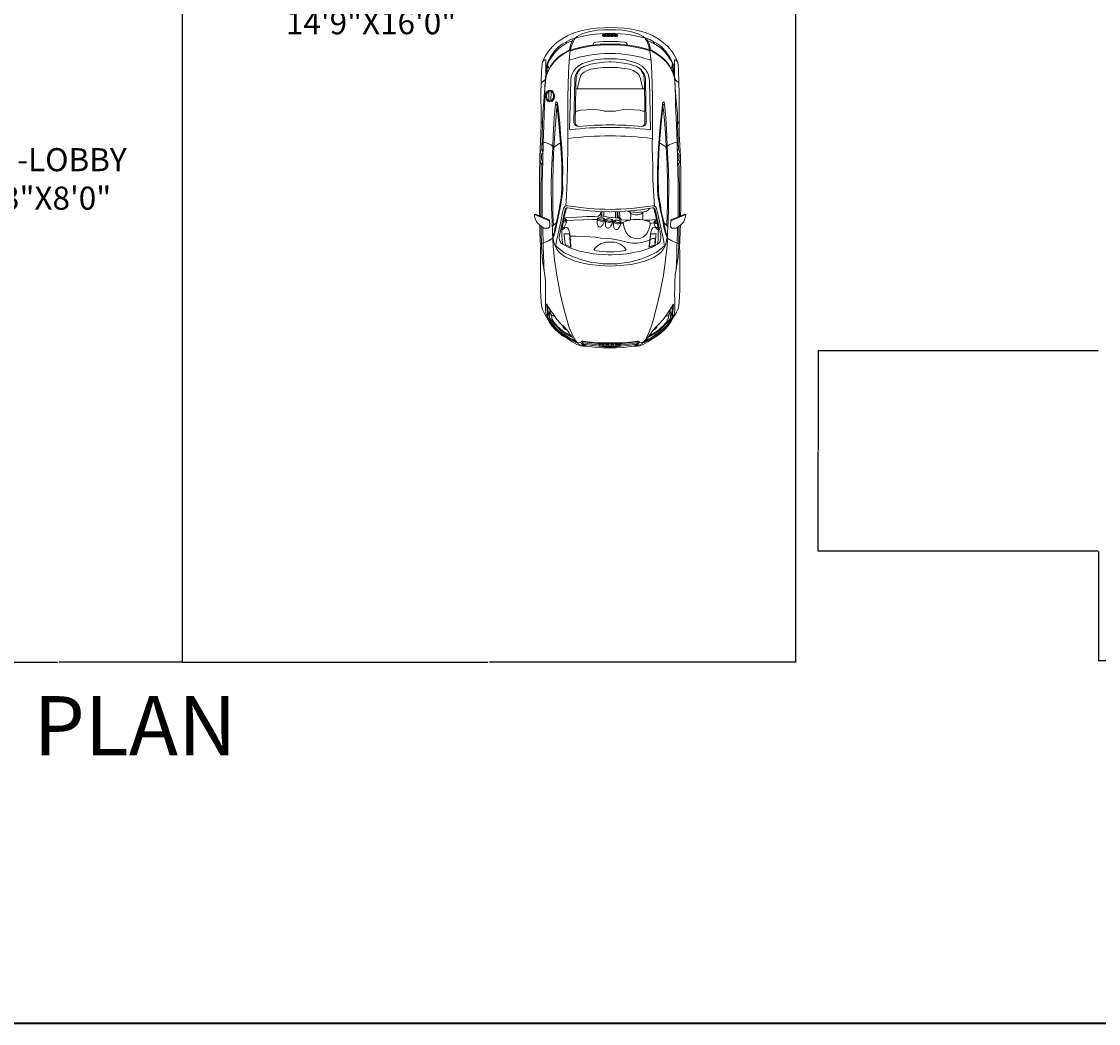
# Model space of a CAD drawing. Units: inches. Extents: x 2215 to 3724, y 1009 to 2124.
# Tile 5 of 11: x 2636 to 2963, y 1009 to 1313. Entities that reach past the tile are written whole.
import ezdxf

# ---------------------------------------------------------------- set-up
doc = ezdxf.new("R2010")
doc.units = ezdxf.units.IN
for name, color, linetype, lineweight in [('A-ANNO-DIMS', 2, 'Continuous', 18), ('A-ANNO-TEXT', 7, 'Continuous', 25), ('A-ANNO-TTLB', 7, 'Continuous', 35), ('A-AREA-IDEN', 7, 'Continuous', 18), ('AUDI', 8, 'Continuous', 13)]:
    doc.layers.add(name, color=color, linetype=linetype, lineweight=lineweight)
doc.styles.get("Standard").update_dxf_attribs({"font": 'arial.ttf'})
doc.dimstyles.get("Standard").update_dxf_attribs({"dimtxt": 0.18, "dimasz": 0.18, "dimexe": 0.18, "dimexo": 0.0625, "dimgap": 0.09, "dimtad": 0, "dimtih": 1, "dimtoh": 1, "dimdec": 4, "dimzin": 0, "dimdsep": 46, "dimtxsty": 'Standard', "dimcen": 0.09, "dimadec": 0, "dimazin": 0, "dimtfac": 1, "dimtdec": 4, "dimtofl": 0, "dimtmove": 0, "dimatfit": 3, "dimfxl": 1, "dimtolj": 1, "dimtzin": 0, "dimarcsym": 0})

# ---------------------------------------------------------------- blocks, each defined once
blk = doc.blocks.new('*D89')
at = {"layer": 'A-ANNO-DIMS', "color": 0, "lineweight": -2, "transparency": 16777216}
for p, q in [((2962.68, 1212.83), (2877.61, 1212.83)), ((2877.79, 1212.65), (2877.79, 1182.6)), ((2877.79, 1152.18), (2877.79, 1182.23)), ((2962.68, 1152), (2877.61, 1152))]:
    blk.add_line(p, q, dxfattribs=at)
at = {"layer": 'A-ANNO-DIMS', "color": 0, "transparency": 16777216}
for points in [[(2877.76, 1212.65), (2877.82, 1212.65), (2877.79, 1212.83)], [(2877.76, 1152.18), (2877.82, 1152.18), (2877.79, 1152)]]:
    blk.add_solid(points, dxfattribs=at)
at = {"layer": 'Defpoints', "color": 0, "transparency": 16777216}
for p in [(2877.79, 1212.83), (2962.74, 1212.83), (2962.74, 1152)]:
    blk.add_point(p, dxfattribs=at)
at = {"layer": 'A-ANNO-DIMS', "color": 0, "transparency": 16777216, "insert": (2877.79, 1182.42), "char_height": 0.18, "attachment_point": 5}
blk.add_mtext('\\A1;60.84', dxfattribs=at)
blk = doc.blocks.new('*D96')
at = {"layer": 'A-ANNO-DIMS', "color": 0, "lineweight": -2, "transparency": 16777216}
for p, q in [((3520.74, 1343.93), (3520.74, 1118.67)), ((2962.74, 1151.93), (2962.74, 1118.67)), ((2962.92, 1118.85), (3241.45, 1118.85)), ((3520.56, 1118.85), (3242.03, 1118.85))]:
    blk.add_line(p, q, dxfattribs=at)
at = {"layer": 'A-ANNO-DIMS', "color": 0, "transparency": 16777216}
for points in [[(2962.92, 1118.88), (2962.92, 1118.82), (2962.74, 1118.85)], [(3520.56, 1118.88), (3520.56, 1118.82), (3520.74, 1118.85)]]:
    blk.add_solid(points, dxfattribs=at)
at = {"layer": 'Defpoints', "color": 0, "transparency": 16777216}
for p in [(3520.74, 1344), (2962.74, 1152), (3520.74, 1118.85)]:
    blk.add_point(p, dxfattribs=at)
at = {"layer": 'A-ANNO-DIMS', "color": 0, "transparency": 16777216, "insert": (3241.74, 1118.85), "char_height": 0.18, "attachment_point": 5}
blk.add_mtext('\\A1;558', dxfattribs=at)
blk = doc.blocks.new('*D99')
at = {"layer": 'A-ANNO-DIMS', "color": 0, "lineweight": -2, "transparency": 16777216}
for p, q in [((2684.84, 1343.93), (2684.84, 1118.22)), ((2609.84, 1151.93), (2609.84, 1118.22)), ((2610.02, 1118.4), (2647.12, 1118.4)), ((2684.66, 1118.4), (2647.56, 1118.4))]:
    blk.add_line(p, q, dxfattribs=at)
at = {"layer": 'A-ANNO-DIMS', "color": 0, "transparency": 16777216}
for points in [[(2610.02, 1118.43), (2610.02, 1118.37), (2609.84, 1118.4)], [(2684.66, 1118.43), (2684.66, 1118.37), (2684.84, 1118.4)]]:
    blk.add_solid(points, dxfattribs=at)
at = {"layer": 'Defpoints', "color": 0, "transparency": 16777216}
for p in [(2684.84, 1344), (2609.84, 1152), (2684.84, 1118.4)]:
    blk.add_point(p, dxfattribs=at)
at = {"layer": 'A-ANNO-DIMS', "color": 0, "transparency": 16777216, "insert": (2647.34, 1118.4), "char_height": 0.18, "attachment_point": 5}
blk.add_mtext('\\A1;75', dxfattribs=at)
blk = doc.blocks.new('*D100')
at = {"layer": 'A-ANNO-DIMS', "color": 0, "lineweight": -2, "transparency": 16777216}
for p, q in [((2684.84, 1343.93), (2684.84, 1118.22)), ((2870.84, 1343.93), (2870.84, 1118.22)), ((2685.02, 1118.4), (2777.56, 1118.4)), ((2870.66, 1118.4), (2778.12, 1118.4))]:
    blk.add_line(p, q, dxfattribs=at)
at = {"layer": 'A-ANNO-DIMS', "color": 0, "transparency": 16777216}
for points in [[(2685.02, 1118.43), (2685.02, 1118.37), (2684.84, 1118.4)], [(2870.66, 1118.43), (2870.66, 1118.37), (2870.84, 1118.4)]]:
    blk.add_solid(points, dxfattribs=at)
at = {"layer": 'Defpoints', "color": 0, "transparency": 16777216}
for p in [(2684.84, 1344), (2870.84, 1344), (2870.84, 1118.4)]:
    blk.add_point(p, dxfattribs=at)
at = {"layer": 'A-ANNO-DIMS', "color": 0, "transparency": 16777216, "insert": (2777.84, 1118.4), "char_height": 0.18, "attachment_point": 5}
blk.add_mtext('\\A1;186', dxfattribs=at)

msp = doc.modelspace()

# ---------------------------------------------------------------- linework, layer by layer
at = {"layer": 'A-ANNO-TTLB'}
msp.add_lwpolyline([(2215.4438, 2124.2681), (3723.6589, 2124.2681), (3723.6589, 1008.7935), (2215.4438, 1008.7935)], close=True, dxfattribs=at)
at = {"layer": 'AUDI'}
for p, q in [((2801.1681, 1305.8265), (2801.323, 1306.5094)), ((2801.4616, 1305.9823), (2801.4475, 1306.5799)), ((2812.3228, 1308.4102), (2812.3228, 1308.6185)), ((2813.5649, 1308.1989), (2813.5649, 1308.4072)), ((2815.7326, 1308.1989), (2815.7326, 1308.4072)), ((2816.9747, 1308.4102), (2816.9747, 1308.6185)), ((2827.8359, 1305.9823), (2827.85, 1306.5799)), ((2828.1294, 1305.8265), (2827.9745, 1306.5094)), ((2804.207, 1292.2283), (2825.0905, 1292.2283)), ((2812.784, 1253.5837), (2812.784, 1255.0226)), ((2816.3282, 1253.0788), (2816.3282, 1255.0178)), ((2817.6075, 1253.179), (2817.377, 1253.179)), ((2826.7535, 1251.4199), (2827.33, 1251.5172)), ((2827.33, 1251.5172), (2828.0282, 1251.5961)), ((2813.1321, 1215.0864), (2813.1321, 1214.8065)), ((2816.0447, 1215.0864), (2816.0447, 1214.8065)), ((2811.4631, 1214.8025), (2811.4631, 1214.5226)), ((2817.7136, 1214.8025), (2817.7136, 1214.5226))]:
    msp.add_line(p, q, dxfattribs=at)
for points in [[(2793.2574, 1253.7096), (2793.2029, 1256.0458), (2793.2029, 1265.8842), (2793.3349, 1271.6287), (2793.6648, 1278.6278), (2793.738, 1281.6587), (2793.738, 1284.4076), (2793.677, 1290.7609), (2793.7685, 1294.304), (2793.8906, 1297.6944), (2794.0127, 1299.7409), (2794.1653, 1300.4435, -0.12683503), (2798.5051, 1306.2746), (2800.0673, 1307.3982), (2801.8248, 1308.4241), (2803.7288, 1309.2058), (2805.0469, 1309.5966), (2806.6579, 1310.0363), (2808.8059, 1310.4271), (2810.5146, 1310.6713), (2814.6488, 1310.8132)], [(2801.2318, 1256.7223), (2801.4068, 1259.7563), (2801.661, 1264.6858), (2801.6928, 1269.1383), (2801.8835, 1274.1632), (2801.8199, 1279.22), (2801.8296, 1289.7659), (2802.0096, 1297.0083), (2802.2323, 1300.7293), (2802.4772, 1303.0689), (2802.6524, 1304.072, -0.10917638), (2804.1487, 1307.7084), (2804.6219, 1308.1481), (2806.1132, 1308.9155), (2808.4993, 1309.6617), (2810.928, 1310.0241), (2812.7815, 1310.1094), (2814.6488, 1310.1094)], [(2836.0402, 1253.7096), (2836.0946, 1256.0458), (2836.0946, 1265.8842), (2835.9626, 1271.6287), (2835.6327, 1278.6278), (2835.5595, 1281.6587), (2835.5595, 1284.4076), (2835.6206, 1290.7609), (2835.529, 1294.304), (2835.4069, 1297.6944), (2835.2848, 1299.7409), (2835.1322, 1300.4435, 0.12683503), (2830.7924, 1306.2746), (2829.2302, 1307.3982), (2827.4727, 1308.4241), (2825.5688, 1309.2058), (2824.2507, 1309.5966), (2822.6396, 1310.0363), (2820.4916, 1310.4271), (2818.7829, 1310.6713), (2814.6488, 1310.8132)], [(2828.0815, 1256.4487), (2827.8908, 1259.7563), (2827.6365, 1264.6858), (2827.6047, 1269.1383), (2827.414, 1274.1632), (2827.4776, 1279.22), (2827.468, 1289.7659), (2827.2879, 1297.0083), (2827.0652, 1300.7293), (2826.8203, 1303.0689), (2826.6451, 1304.072, 0.10917638), (2825.1488, 1307.7084), (2824.6757, 1308.1481), (2823.1843, 1308.9155), (2820.7982, 1309.6617), (2818.3695, 1310.0241), (2816.516, 1310.1094), (2814.6488, 1310.1094)], [(2828.0657, 1256.7223), (2827.8908, 1259.7563), (2827.6365, 1264.6858), (2827.6047, 1269.1383), (2827.414, 1274.1632), (2827.4776, 1279.22), (2827.468, 1289.7659), (2827.2879, 1297.0083), (2827.0652, 1300.7293), (2826.8203, 1303.0689), (2826.6451, 1304.072, 0.10917638), (2825.1488, 1307.7084), (2824.6757, 1308.1481), (2823.1843, 1308.9155), (2820.7982, 1309.6617), (2818.3695, 1310.0241), (2816.516, 1310.1094), (2814.6488, 1310.1094)], [(2802.6416, 1307.2132, -0.1536904), (2826.6529, 1307.2309)], [(2810.3678, 1306.4047, -0.05356625), (2818.9097, 1306.4131, -0.05356625)], [(2802.603, 1303.7893, -0.14863541), (2826.6914, 1303.8068)], [(2802.6416, 1304.01, -0.1536904), (2826.6529, 1304.0276)], [(2802.2669, 1300.8894, -0.16706429), (2827.0472, 1300.9013, -0.16706429)], [(2802.5474, 1279.8089, -0.4622712), (2802.3789, 1280.0174), (2802.7384, 1294.8022, -0.18047602), (2804.1724, 1298.3779), (2804.9717, 1299.1307), (2806.2882, 1299.9305), (2808.2395, 1300.5421), (2810.0261, 1301.0597), (2812.7105, 1301.3722), (2814.6488, 1301.3722)], [(2805.0527, 1280.8316, -0.40402709), (2803.6614, 1282.0372), (2803.9118, 1294.9627, -0.22167644), (2805.5552, 1298.3163, -0.05999808), (2806.6597, 1299.0072), (2808.7671, 1299.718), (2810.4955, 1300.0734), (2812.816, 1300.334), (2814.3314, 1300.3814), (2814.6488, 1300.3814)], [(2826.7501, 1279.8089, 0.4622712), (2826.9186, 1280.0174), (2826.5592, 1294.8022, 0.18047602), (2825.1251, 1298.3779), (2824.3258, 1299.1307), (2823.0093, 1299.9305), (2821.0581, 1300.5421), (2819.2714, 1301.0597), (2816.5871, 1301.3722), (2814.6488, 1301.3722)], [(2824.2448, 1280.8316, 0.40402709), (2825.6361, 1282.0372), (2825.3858, 1294.9627, 0.22167644), (2823.7423, 1298.3163, 0.05999808), (2822.6378, 1299.0072), (2820.5305, 1299.718), (2818.802, 1300.0734), (2816.4816, 1300.334), (2814.9662, 1300.3814), (2814.6488, 1300.3814)], [(2805.9218, 1298.5875, 0.17077992), (2804.3629, 1295.619), (2804.2209, 1293.1548), (2804.1262, 1286.8287), (2804.0773, 1282.1936, 0.32699174), (2805.0527, 1280.8316, 1.80630344)], [(2808.7835, 1298.1873, -0.05874602), (2814.6488, 1298.7307, -0.04602302)], [(2820.5141, 1298.1873, 0.05874602), (2814.6488, 1298.7307, 0.04602302)], [(2823.3757, 1298.5875, -0.17077992), (2824.9346, 1295.619), (2825.0767, 1293.1548), (2825.1714, 1286.8287), (2825.2203, 1282.1936, -0.32699174), (2824.2448, 1280.8316, -1.80630344)], [(2802.5474, 1279.8089, -0.0615843), (2826.7583, 1279.8093, -0.0615843)], [(2805.0527, 1280.8316, -0.04880378), (2824.2662, 1280.8307, -0.04880378)], [(2801.8461, 1277.141, -0.06516086), (2827.4515, 1277.1425, -4.49164968)], [(2794.0848, 1269.347), (2794.1591, 1270.5362), (2794.1591, 1270.5362), (2794.0319, 1270.5275), (2793.9329, 1270.6018), (2793.8586, 1270.8248, -0.17711693), (2793.9081, 1272.5342), (2794.0113, 1272.6168), (2794.1459, 1272.6956), (2794.1459, 1272.6956), (2794.2086, 1272.7411), (2794.1839, 1273.3605), (2794.1096, 1273.8808), (2793.8338, 1273.8225), (2793.7638, 1273.6805, 0.20734628), (2793.7885, 1269.4937), (2793.809, 1269.4374), (2793.9824, 1269.3136), (2794.0848, 1269.347)], [(2835.2127, 1269.347), (2835.1384, 1270.5362), (2835.1384, 1270.5362), (2835.2656, 1270.5275), (2835.3647, 1270.6018), (2835.439, 1270.8248, 0.17711693), (2835.3894, 1272.5342), (2835.2862, 1272.6168), (2835.1517, 1272.6956), (2835.1517, 1272.6956), (2835.0889, 1272.7411), (2835.1137, 1273.3605), (2835.188, 1273.8808), (2835.4637, 1273.8225), (2835.5337, 1273.6805, -0.20734628), (2835.509, 1269.4937), (2835.4885, 1269.4374), (2835.3151, 1269.3136), (2835.2127, 1269.347)], [(2798.1177, 1244.3211), (2798.4791, 1246.5332), (2799.0555, 1249.1864), (2799.7759, 1252.474), (2800.2659, 1254.6945), (2800.5541, 1255.9346, -0.36424732), (2801.7068, 1256.7997, 0.04353666), (2814.6488, 1255.6808)], [(2814.6488, 1241.9147), (2814.0256, 1241.9147), (2811.5597, 1242.0028), (2809.5341, 1242.2231), (2807.5525, 1242.5756), (2805.3389, 1243.0544), (2803.5544, 1243.5969), (2802.1313, 1244.1393), (2800.8663, 1244.7949), (2800.2338, 1245.1565), (2799.8272, 1245.4504), (2799.4884, 1245.9025), (2799.3302, 1246.4224), (2799.2399, 1247.0101), (2799.2625, 1247.8464), (2800.9793, 1255.5995, -0.41343093), (2801.7925, 1256.1194), (2802.9967, 1255.9594), (2805.4544, 1255.5616), (2808.6349, 1255.2361), (2811.5263, 1255.0553), (2814.3093, 1254.9829)], [(2831.1798, 1244.3211), (2830.8185, 1246.5332), (2830.2421, 1249.1864), (2829.5216, 1252.474), (2829.0317, 1254.6945), (2828.7435, 1255.9346, 0.36424732), (2827.5907, 1256.7997, -0.04353666), (2814.6488, 1255.6808)], [(2814.6488, 1241.9147), (2815.2719, 1241.9147), (2817.7379, 1242.0028), (2819.7635, 1242.2231), (2821.7451, 1242.5756), (2823.9586, 1243.0544), (2825.7431, 1243.5969), (2827.1662, 1244.1393), (2828.4312, 1244.7949), (2829.0637, 1245.1565), (2829.4703, 1245.4504), (2829.8092, 1245.9025), (2829.9673, 1246.4224), (2830.0576, 1247.0101), (2830.035, 1247.8464), (2828.3183, 1255.5995, 0.41343093), (2827.5051, 1256.1194), (2826.3008, 1255.9594), (2823.8431, 1255.5616), (2820.6626, 1255.2361), (2817.7712, 1255.0553), (2814.9882, 1254.9829)], [(2819.8124, 1255.1829), (2820.1661, 1255.0256, 0.09257149), (2825.552, 1255.0256), (2826.1747, 1255.4617), (2826.6536, 1256.0063)], [(2822.6407, 1254.0124, -0.11496238), (2821.068, 1254.3714), (2820.6633, 1254.7141), (2820.5953, 1254.952)], [(2822.6407, 1254.0124, 0.11496238), (2824.2133, 1254.3714), (2824.618, 1254.7141), (2824.6678, 1254.8882)], [(2800.1147, 1250.0559, 0.30781353), (2800.8353, 1250.464), (2801.076, 1250.8446), (2801.3322, 1251.4676), (2801.4175, 1251.9726), (2801.4719, 1252.375), (2801.4665, 1252.5116), (2801.318, 1252.7381, 0.10075057), (2800.6404, 1252.9063, 0.03883263)], [(2810.7936, 1252.7669), (2810.7655, 1252.4293), (2810.7515, 1251.9791), (2810.7655, 1251.4726), (2810.8358, 1250.9661, 0.69697601), (2812.1856, 1250.6706), (2812.4668, 1251.0223), (2812.7901, 1251.6133), (2812.9307, 1252.1057), (2813.0292, 1252.4996), (2813.0389, 1252.636), (2812.7761, 1252.978, 0.1146222), (2811.2295, 1253.1609), (2811.0327, 1253.0764), (2810.8499, 1252.9357), (2810.7936, 1252.7669)], [(2813.2485, 1252.4241), (2813.2204, 1252.0865), (2813.2064, 1251.6363), (2813.2204, 1251.1298), (2813.2907, 1250.6233, 0.69697601), (2814.6405, 1250.3279), (2814.9217, 1250.6796), (2815.245, 1251.2705), (2815.3856, 1251.7629), (2815.4841, 1252.1568), (2815.4938, 1252.2932), (2815.231, 1252.6352, 0.1146222), (2813.6844, 1252.8181), (2813.4876, 1252.7337), (2813.3048, 1252.593), (2813.2485, 1252.4241)], [(2815.7546, 1251.9833), (2815.7265, 1251.6456), (2815.7124, 1251.1954), (2815.7265, 1250.689), (2815.7968, 1250.1825, 0.69697601), (2817.1465, 1249.887), (2817.4277, 1250.2387), (2817.7511, 1250.8296), (2817.8917, 1251.3221), (2817.9901, 1251.716), (2817.9998, 1251.8524), (2817.737, 1252.1944, 0.1146222), (2816.1904, 1252.3773), (2815.9936, 1252.2928), (2815.8108, 1252.1521), (2815.7546, 1251.9833)], [(2818.5801, 1251.7302), (2818.6793, 1250.9607), (2819.0018, 1249.8437), (2819.5475, 1248.7019, 0.61645483), (2826.0961, 1248.9253), (2826.5178, 1249.8686), (2826.7659, 1250.9111), (2826.7411, 1251.9287, 0.20084491), (2818.5801, 1251.7302, 3.44889889)], [(2829.124, 1250.3307, -0.43942644), (2828.5577, 1250.1994), (2828.3282, 1250.4647), (2828.1346, 1250.9355), (2828.0492, 1251.4405), (2827.9948, 1251.8429), (2828.0002, 1251.9795), (2828.1487, 1252.206, -0.09128884), (2828.7608, 1252.3702, -0.09128884)], [(2802.4871, 1247.6), (2804.1652, 1247.6), (2807.023, 1247.4833), (2810.2308, 1247.2498), (2812.3887, 1246.8996), (2815.0716, 1246.7246), (2817.7544, 1246.1993), (2819.3292, 1245.7908, 0.12760018), (2824.9865, 1245.7908), (2826.248, 1246.2818), (2826.8913, 1246.5577), (2827.5039, 1246.8182), (2827.9021, 1246.8948), (2828.1624, 1246.8948), (2828.2696, 1246.6343), (2828.2006, 1245.3967)], [(2814.6488, 1242.8529), (2813.5471, 1242.8529), (2811.3476, 1242.9718), (2810.5512, 1243.1377), (2810.0676, 1243.2399), (2809.8861, 1243.367), (2809.8316, 1243.4942), (2809.8679, 1243.6486, -0.25546602), (2814.6488, 1245.7741, -2.79521639)], [(2814.6488, 1242.8529), (2815.7504, 1242.8529), (2817.95, 1242.9718), (2818.7463, 1243.1377), (2819.2299, 1243.2399), (2819.4115, 1243.367), (2819.4659, 1243.4942), (2819.4296, 1243.6486, 0.25546602), (2814.6488, 1245.7741, 2.79521639)], [(2800.2416, 1220.472, 0.27931409), (2801.6606, 1219.0017, 0.27931409)], [(2829.056, 1220.472, -0.27931409), (2827.637, 1219.0017, -0.27931409)]]:
    msp.add_lwpolyline(points, format="xyb", dxfattribs=at)
for points in [[(2802.6416, 1307.2132), (2801.5459, 1306.6356), (2800.0836, 1305.8074), (2798.9524, 1304.8411), (2797.7385, 1303.5987), (2796.6073, 1301.9146), (2795.9175, 1300.6447), (2795.5313, 1299.8716), (2795.3657, 1299.0158), (2795.3657, 1297.9391), (2795.3382, 1296.7243), (2795.3206, 1296.2338)], [(2803.2085, 1306.7744), (2802.37, 1306.4643), (2800.8669, 1305.6667), (2799.1588, 1304.5272), (2798.0656, 1303.4333), (2797.0635, 1302.1571), (2796.3575, 1301.0177), (2795.9704, 1300.3112), (2795.7654, 1299.7871), (2795.6743, 1299.1262), (2795.606, 1298.0323), (2795.606, 1297.2229)], [(2803.5853, 1307.4984), (2803.2565, 1306.8841), (2802.6771, 1305.5589), (2802.4564, 1304.5926), (2802.3309, 1304.04)], [(2810.3678, 1306.4047), (2809.7673, 1306.1511), (2809.5021, 1305.8193), (2809.4181, 1305.5168)], [(2814.6488, 1308.4261), (2814.6488, 1308.2178)], [(2818.9097, 1306.4131), (2819.5302, 1306.1511), (2819.7954, 1305.8193), (2819.8774, 1305.5241)], [(2825.7122, 1307.4984), (2826.041, 1306.8841), (2826.6204, 1305.5589), (2826.8411, 1304.5926), (2826.9667, 1304.04)], [(2826.089, 1306.7744), (2826.9276, 1306.4643), (2828.4307, 1305.6667), (2830.1388, 1304.5272), (2831.2319, 1303.4333), (2832.234, 1302.1571), (2832.94, 1301.0177), (2833.3272, 1300.3112), (2833.5321, 1299.7871), (2833.6232, 1299.1262), (2833.6915, 1298.0323), (2833.6915, 1297.2229)], [(2826.656, 1307.2132), (2827.7516, 1306.6356), (2829.2139, 1305.8074), (2830.3451, 1304.8411), (2831.559, 1303.5987), (2832.6902, 1301.9146), (2833.38, 1300.6447), (2833.7662, 1299.8716), (2833.9318, 1299.0158), (2833.9318, 1297.9391), (2833.9594, 1296.7243), (2833.9769, 1296.2338)], [(2802.3309, 1304.04), (2801.999, 1303.8657), (2800.4359, 1302.9951), (2798.9466, 1301.8737), (2797.6637, 1300.6194), (2796.5697, 1299.1071), (2795.6496, 1297.3128), (2795.3361, 1296.6656)], [(2802.6416, 1304.01), (2801.999, 1303.6724), (2800.4359, 1302.8018), (2798.9466, 1301.6804), (2797.6637, 1300.4262), (2796.5697, 1298.9138), (2795.6496, 1297.1195), (2795.4127, 1296.6305)], [(2826.656, 1304.01), (2827.2985, 1303.6724), (2828.8616, 1302.8018), (2830.3509, 1301.6804), (2831.6338, 1300.4262), (2832.7278, 1298.9138), (2833.648, 1297.1195), (2833.8848, 1296.6305)], [(2826.9667, 1304.04), (2827.2985, 1303.8657), (2828.8616, 1302.9951), (2830.3509, 1301.8737), (2831.6338, 1300.6194), (2832.7278, 1299.1071), (2833.648, 1297.3128), (2833.9615, 1296.6656)], [(2794.0225, 1253.3989), (2794.0225, 1259.1275), (2794.0225, 1263.7106), (2794.2045, 1270.4183), (2794.3562, 1275.8513), (2794.5601, 1281.2664), (2794.8027, 1287.2882), (2794.8351, 1289.1349), (2794.9036, 1293.0363), (2795.1268, 1296.5975), (2795.1208, 1298.8552), (2795.1247, 1300.5002)], [(2795.1247, 1300.5002), (2795.1198, 1300.9076), (2795.0199, 1301.0327), (2794.8325, 1301.0327), (2794.6826, 1300.9701), (2794.5202, 1300.8076), (2794.2953, 1300.5451), (2794.1482, 1300.3644)], [(2796.2643, 1298.3184), (2796.0387, 1298.6248), (2795.8565, 1298.9438), (2795.7882, 1299.3996), (2795.7654, 1300.0377), (2795.7978, 1300.405)], [(2833.0332, 1298.3184), (2833.2588, 1298.6248), (2833.441, 1298.9438), (2833.5094, 1299.3996), (2833.5321, 1300.0377), (2833.4997, 1300.405)], [(2835.275, 1253.3989), (2835.275, 1259.1275), (2835.275, 1263.7106), (2835.093, 1270.4183), (2834.9413, 1275.8513), (2834.7374, 1281.2664), (2834.4948, 1287.2882), (2834.4624, 1289.1349), (2834.3939, 1293.0363), (2834.1707, 1296.5975), (2834.1767, 1298.8552), (2834.1729, 1300.5002)], [(2834.1729, 1300.5002), (2834.1777, 1300.9076), (2834.2777, 1301.0327), (2834.465, 1301.0327), (2834.6149, 1300.9701), (2834.7773, 1300.8076), (2835.0022, 1300.5451), (2835.1494, 1300.3644)], [(2795.4127, 1296.6305), (2795.1529, 1295.5105), (2794.7931, 1291.2503), (2794.5732, 1288.5302), (2794.2534, 1284.83), (2794.1758, 1281.7327), (2793.9015, 1273.8368)], [(2808.7835, 1298.1873), (2807.6917, 1297.7784), (2806.8183, 1297.2977), (2805.9231, 1296.5548), (2805.4427, 1295.3749), (2804.9841, 1293.4959), (2804.744, 1292.4034)], [(2820.5141, 1298.1873), (2821.6058, 1297.7784), (2822.4792, 1297.2977), (2823.3745, 1296.5548), (2823.8548, 1295.3749), (2824.3134, 1293.4959), (2824.5536, 1292.4034)], [(2833.8848, 1296.6305), (2834.1447, 1295.5105), (2834.5045, 1291.2503), (2834.7243, 1288.5302), (2835.0441, 1284.83), (2835.1217, 1281.7327), (2835.396, 1273.8368)], [(2793.7575, 1293.8775), (2794.0335, 1294.2504), (2794.4333, 1294.5705), (2795.0347, 1295.1271)], [(2835.54, 1293.8775), (2835.264, 1294.2504), (2834.8642, 1294.5705), (2834.2629, 1295.1271)], [(2796.0631, 1288.6785), (2796.113, 1291.4956)], [(2796.6847, 1288.6366), (2796.7357, 1291.5178)], [(2793.5439, 1245.4164), (2793.8393, 1245.332), (2794.3207, 1245.3922), (2794.8323, 1245.603), (2795.9457, 1246.1149), (2797.0892, 1246.8677), (2797.36, 1247.1688), (2797.6496, 1247.8053), (2798.2007, 1249.9217), (2798.7904, 1252.7692), (2799.4313, 1255.6295), (2799.6876, 1257.0533), (2799.803, 1257.8742), (2800.0289, 1259.2221), (2800.2705, 1261.4822), (2800.2377, 1264.304), (2800.2705, 1267.6179), (2800.2134, 1270.1202), (2800.0094, 1274.4449), (2799.657, 1278.5282), (2799.3788, 1281.9063), (2799.0806, 1284.577), (2798.7542, 1287.4268), (2798.6059, 1288.0799), (2798.3389, 1288.258), (2798.2228, 1288.1652), (2798.1016, 1287.5752), (2797.7159, 1283.4786), (2797.4193, 1278.0758), (2797.3006, 1274.6323), (2797.0929, 1271.0996), (2796.915, 1267.4483), (2796.826, 1262.9657), (2796.9205, 1256.2273), (2797.0628, 1251.8117), (2797.2051, 1248.7256), (2797.2645, 1246.3311), (2797.3594, 1244.527), (2797.8338, 1240.3488), (2798.4981, 1235.6958), (2799.5419, 1230.1882), (2800.5383, 1225.9626), (2801.5821, 1221.9744), (2802.2526, 1219.8195), (2803.0118, 1218.0152), (2803.8184, 1216.3535), (2804.246, 1215.773), (2804.6865, 1215.2897)], [(2797.2358, 1247.4884), (2797.7178, 1248.7183), (2798.0139, 1250.146), (2798.3638, 1251.816), (2799.1175, 1255.183), (2799.3598, 1256.9877), (2799.7635, 1259.1156), (2799.925, 1260.5702), (2799.9789, 1262.0516), (2800.0327, 1264.0449), (2800.0437, 1265.9342), (2800.0139, 1269.3494), (2799.8516, 1272.8564), (2799.5596, 1276.9803), (2799.1377, 1281.7537), (2798.8132, 1284.6438), (2798.6185, 1286.9493), (2798.5234, 1287.4407), (2798.4857, 1287.5139), (2798.4092, 1287.542), (2798.3224, 1287.4926), (2798.2901, 1287.3631), (2798.2772, 1287.1431)], [(2798.6075, 1287.0062), (2798.413, 1285.8098), (2798.2747, 1283.7658), (2797.9769, 1280.2558), (2797.7949, 1277.2095), (2797.6129, 1274.4942), (2797.3686, 1269.5528), (2797.284, 1263.5388), (2797.284, 1257.1012), (2797.3263, 1254.0942)], [(2835.7536, 1245.4164), (2835.4583, 1245.332), (2834.9768, 1245.3922), (2834.4652, 1245.603), (2833.3519, 1246.1149), (2832.2084, 1246.8677), (2831.9375, 1247.1688), (2831.648, 1247.8053), (2831.0968, 1249.9217), (2830.5072, 1252.7692), (2829.8663, 1255.6295), (2829.6099, 1257.0533), (2829.4946, 1257.8742), (2829.2686, 1259.2221), (2829.027, 1261.4822), (2829.0598, 1264.304), (2829.027, 1267.6179), (2829.0841, 1270.1202), (2829.2881, 1274.4449), (2829.6406, 1278.5282), (2829.9188, 1281.9063), (2830.217, 1284.577), (2830.5433, 1287.4268), (2830.6916, 1288.0799), (2830.9586, 1288.258), (2831.0747, 1288.1652), (2831.1959, 1287.5752), (2831.5816, 1283.4786), (2831.8783, 1278.0758), (2831.9969, 1274.6323), (2832.2046, 1271.0996), (2832.3826, 1267.4483), (2832.4716, 1262.9657), (2832.3771, 1256.2273), (2832.2347, 1251.8117), (2832.0924, 1248.7256), (2832.0331, 1246.3311), (2831.9382, 1244.527), (2831.4637, 1240.3488), (2830.7995, 1235.6958), (2829.7556, 1230.1882), (2828.7592, 1225.9626), (2827.7154, 1221.9744), (2827.0449, 1219.8195), (2826.2858, 1218.0152), (2825.4792, 1216.3535), (2825.0516, 1215.773), (2824.611, 1215.2897)], [(2832.0617, 1247.4884), (2831.5797, 1248.7183), (2831.2836, 1250.146), (2830.9337, 1251.816), (2830.18, 1255.183), (2829.9378, 1256.9877), (2829.534, 1259.1156), (2829.3725, 1260.5702), (2829.3187, 1262.0516), (2829.2648, 1264.0449), (2829.2539, 1265.9342), (2829.2837, 1269.3494), (2829.4459, 1272.8564), (2829.738, 1276.9803), (2830.1598, 1281.7537), (2830.4843, 1284.6438), (2830.679, 1286.9493), (2830.7741, 1287.4407), (2830.8118, 1287.5139), (2830.8884, 1287.542), (2830.9751, 1287.4926), (2831.0074, 1287.3631), (2831.0204, 1287.1431)], [(2830.69, 1287.0062), (2830.8845, 1285.8098), (2831.0228, 1283.7658), (2831.3206, 1280.2558), (2831.5026, 1277.2095), (2831.6846, 1274.4942), (2831.9289, 1269.5528), (2832.0135, 1263.5388), (2832.0135, 1257.1012), (2831.9712, 1254.0942)], [(2804.1121, 1285.4911), (2804.744, 1285.4911), (2805.6741, 1285.7516), (2807.5715, 1285.9005), (2809.6922, 1285.9378), (2810.9571, 1285.8261), (2812.2964, 1285.6772), (2813.0033, 1285.4911), (2814.6488, 1285.4911)], [(2825.1855, 1285.4911), (2824.5535, 1285.4911), (2823.6234, 1285.7516), (2821.726, 1285.9005), (2819.6054, 1285.9378), (2818.3404, 1285.8261), (2817.0011, 1285.6772), (2816.2942, 1285.4911), (2814.6488, 1285.4911)], [(2794.1758, 1281.732), (2793.9503, 1282.0295), (2793.738, 1282.5542)], [(2835.1217, 1281.732), (2835.3473, 1282.0295), (2835.5595, 1282.5542)], [(2799.6358, 1275.9035), (2799.1385, 1275.605), (2798.3306, 1275.0777), (2797.8036, 1274.6383), (2797.6114, 1274.4642), (2797.3996, 1274.5504), (2797.2064, 1274.8316), (2796.7321, 1275.2183), (2796.0295, 1275.5698), (2795.2215, 1275.8686), (2794.6834, 1275.94), (2794.3563, 1275.9055), (2794.2588, 1275.7275), (2794.0809, 1275.3715), (2793.9456, 1275.1047)], [(2829.6617, 1275.9035), (2830.159, 1275.605), (2830.967, 1275.0777), (2831.4939, 1274.6383), (2831.6861, 1274.4642), (2831.8979, 1274.5504), (2832.0911, 1274.8316), (2832.5654, 1275.2183), (2833.268, 1275.5698), (2834.076, 1275.8686), (2834.6141, 1275.94), (2834.9412, 1275.9055), (2835.0388, 1275.7275), (2835.2167, 1275.3715), (2835.352, 1275.1047)], [(2793.8507, 1272.3748), (2793.8035, 1271.0151)], [(2835.4468, 1272.3748), (2835.4941, 1271.0151)], [(2793.7534, 1269.5752), (2793.7124, 1268.3943), (2793.6517, 1259.9453), (2793.6517, 1253.5495)], [(2835.5441, 1269.5752), (2835.5851, 1268.3943), (2835.6459, 1259.9453), (2835.6459, 1253.5495)], [(2796.3721, 1250.4291), (2796.2558, 1252.4921), (2792.0284, 1254.2087), (2791.687, 1254.1703), (2791.7765, 1253.3731), (2792.2842, 1251.9308), (2793.3229, 1250.894), (2794.5762, 1249.9969), (2795.879, 1249.9725), (2796.3721, 1250.4291)], [(2791.687, 1254.1703), (2796.2699, 1252.2423)], [(2797.3263, 1254.0942), (2797.4487, 1250.7872)], [(2801.3902, 1256.0853), (2801.1904, 1255.2857), (2800.7576, 1253.512), (2800.5103, 1252.2333), (2800.2011, 1250.4597), (2800.0156, 1249.5935), (2800.0362, 1248.5211), (2800.0569, 1247.428), (2800.1187, 1246.4587), (2800.2011, 1245.6131), (2800.3319, 1245.1004)], [(2811.814, 1253.4604), (2811.8964, 1253.7902), (2811.8964, 1254.0993), (2811.814, 1254.1405), (2811.6286, 1254.1405), (2811.3402, 1253.8314), (2811.1343, 1253.6459), (2810.0461, 1253.5407), (2807.7063, 1253.5407), (2804.5426, 1253.3098), (2801.2704, 1253.0742), (2800.6635, 1253.0256)], [(2811.7439, 1254.1405), (2811.7992, 1255.0482)], [(2812.1407, 1253.6737), (2812.1576, 1255.0389)], [(2814.3093, 1254.9829), (2814.6488, 1254.9829)], [(2816.8147, 1253.0227), (2816.7899, 1255.0298)], [(2817.1296, 1252.9865), (2817.0047, 1255.0353)], [(2818.0643, 1252.5119), (2817.6075, 1253.179), (2817.4836, 1255.0478)], [(2820.8274, 1252.4474), (2820.9485, 1254.4725)], [(2824.5997, 1252.5142), (2824.5295, 1254.6391)], [(2827.9073, 1256.0853), (2828.1071, 1255.2857), (2828.5399, 1253.512), (2828.7872, 1252.2333), (2829.0964, 1250.4597), (2829.2819, 1249.5935), (2829.2613, 1248.5211), (2829.2407, 1247.428), (2829.1788, 1246.4587), (2829.0964, 1245.6131), (2828.9656, 1245.1004)], [(2831.9712, 1254.0942), (2831.8488, 1250.7872)], [(2832.9254, 1250.4291), (2833.0418, 1252.4921), (2837.2691, 1254.2087), (2837.6106, 1254.1703), (2837.5211, 1253.3731), (2837.0134, 1251.9308), (2835.9747, 1250.894), (2834.7213, 1249.9969), (2833.4185, 1249.9725), (2832.9254, 1250.4291)], [(2837.6106, 1254.1703), (2833.0277, 1252.2423)], [(2807.0234, 1214.2115), (2806.3474, 1214.2115), (2805.5514, 1214.341), (2804.5878, 1214.7543), (2803.1883, 1215.4889), (2801.7888, 1216.3843), (2800.4352, 1217.1878), (2799.1504, 1218.198), (2798.0032, 1219.2311), (2796.9929, 1220.3745), (2796.2026, 1221.5365), (2795.4123, 1222.9567), (2794.6382, 1224.2801), (2794.1382, 1225.2969), (2793.8479, 1226.4266), (2793.6066, 1229.1963), (2793.5372, 1231.343), (2793.5372, 1243.1503), (2793.5653, 1243.8934), (2793.6479, 1244.6365), (2793.4828, 1245.8751), (2793.3591, 1249.3429), (2793.3229, 1250.894)], [(2797.1278, 1250.4018), (2797.6101, 1250.981), (2798.1485, 1251.4927), (2798.3113, 1251.5651)], [(2801.4653, 1252.3262), (2803.6405, 1252.3806), (2806.5376, 1252.4623), (2809.3531, 1252.5848), (2810.9036, 1252.6256)], [(2817.1296, 1252.9865), (2816.0569, 1253.11), (2814.9452, 1253.2381), (2814.1414, 1253.3573), (2813.1734, 1253.5222), (2812.3907, 1253.6459), (2811.8346, 1253.7077)], [(2820.6091, 1252.4014), (2819.2527, 1252.3876), (2818.0916, 1252.5068), (2817.6152, 1252.5962), (2817.4366, 1252.7451), (2817.377, 1253.0431), (2817.377, 1253.2516), (2817.1134, 1253.2516)], [(2818.6663, 1251.3986), (2817.9337, 1251.4902)], [(2818.5801, 1251.7302), (2817.9998, 1251.8524)], [(2822.2741, 1214.2115), (2822.9501, 1214.2115), (2823.7462, 1214.341), (2824.7098, 1214.7543), (2826.1093, 1215.4889), (2827.5088, 1216.3843), (2828.8624, 1217.1878), (2830.1472, 1218.198), (2831.2943, 1219.2311), (2832.3047, 1220.3745), (2833.095, 1221.5365), (2833.8852, 1222.9567), (2834.6594, 1224.2801), (2835.1593, 1225.2969), (2835.4496, 1226.4266), (2835.6909, 1229.1963), (2835.7604, 1231.343), (2835.7604, 1243.1503), (2835.7322, 1243.8934), (2835.6497, 1244.6365), (2835.8147, 1245.8751), (2835.9385, 1249.3429), (2835.9746, 1250.894)], [(2828.6959, 1252.7056), (2827.5893, 1252.5068), (2826.7285, 1252.4436), (2825.1181, 1252.4472), (2824.9763, 1252.4458)], [(2826.7411, 1251.9287), (2825.1181, 1252.4472), (2824.9763, 1252.4458)], [(2832.1697, 1250.4018), (2831.6874, 1250.981), (2831.1491, 1251.4927), (2830.9863, 1251.5651)], [(2794.6526, 1237.327), (2794.2907, 1239.3999), (2794.0198, 1241.297), (2793.8995, 1243.0134), (2793.8092, 1244.4888), (2793.8393, 1245.874), (2793.7791, 1248.3131), (2793.7791, 1250.5675)], [(2795.7648, 1222.8209), (2795.4705, 1223.3969), (2795.2448, 1223.9805), (2795.1507, 1224.3759), (2795.0566, 1225.242), (2795.0378, 1226.8046), (2795.019, 1228.3861), (2795.0754, 1229.817), (2795.019, 1231.775), (2795.0378, 1233.9213), (2794.9061, 1235.7099), (2794.6051, 1237.6303), (2794.5314, 1239.2795), (2794.411, 1241.8089), (2794.3809, 1244.3383), (2794.3207, 1245.7234), (2794.2305, 1249.1562), (2794.2305, 1250.2444)], [(2800.019, 1249.4163), (2800.3866, 1249.7172), (2800.8194, 1250.0679), (2801.3141, 1250.1916), (2801.7057, 1250.0885), (2802.0354, 1249.7172), (2802.2003, 1249.1191), (2802.427, 1248.2942), (2802.6125, 1246.1493), (2802.7774, 1244.5819), (2802.7908, 1243.888)], [(2800.7164, 1248.2942), (2802.2415, 1248.2942), (2802.3034, 1248.1292), (2802.4683, 1246.9537), (2802.5713, 1245.6131), (2802.6744, 1244.685), (2802.6744, 1244.4169), (2802.6125, 1244.3138), (2802.4476, 1244.3757), (2801.582, 1244.7469), (2800.9843, 1245.0562), (2800.8813, 1246.0256), (2800.737, 1247.8817), (2800.7164, 1248.2942)], [(2829.2785, 1249.4163), (2828.9109, 1249.7172), (2828.4781, 1250.0679), (2827.9834, 1250.1916), (2827.5918, 1250.0885), (2827.2621, 1249.7172), (2827.0972, 1249.1191), (2826.8705, 1248.2942), (2826.685, 1246.1493), (2826.5201, 1244.5819), (2826.5068, 1243.888)], [(2828.5811, 1248.2942), (2827.056, 1248.2942), (2826.9941, 1248.1292), (2826.8293, 1246.9537), (2826.7262, 1245.6131), (2826.6232, 1244.685), (2826.6232, 1244.4169), (2826.685, 1244.3138), (2826.8499, 1244.3757), (2827.7155, 1244.7469), (2828.3132, 1245.0562), (2828.4163, 1246.0256), (2828.5605, 1247.8817), (2828.5811, 1248.2942)], [(2833.5327, 1222.8209), (2833.827, 1223.3969), (2834.0528, 1223.9805), (2834.1469, 1224.3759), (2834.2409, 1225.242), (2834.2597, 1226.8046), (2834.2786, 1228.3861), (2834.2221, 1229.817), (2834.2786, 1231.775), (2834.2597, 1233.9213), (2834.3914, 1235.7099), (2834.6925, 1237.6303), (2834.7662, 1239.2795), (2834.8865, 1241.8089), (2834.9166, 1244.3383), (2834.9768, 1245.7234), (2835.0671, 1249.1562), (2835.0671, 1250.2444)], [(2834.6449, 1237.327), (2835.0069, 1239.3999), (2835.2777, 1241.297), (2835.3981, 1243.0134), (2835.4883, 1244.4888), (2835.4583, 1245.874), (2835.5184, 1248.3131), (2835.5184, 1250.5675)], [(2814.6488, 1238.5088), (2811.5799, 1238.6377), (2808.3047, 1238.9827), (2806.0294, 1239.4312), (2804.0643, 1239.9832), (2802.375, 1240.6386), (2801.2373, 1241.1906), (2800.0307, 1241.9496), (2799.2033, 1242.674), (2798.5138, 1243.4675), (2798.0656, 1244.4335), (2797.8932, 1244.8474), (2797.6174, 1245.7444), (2797.4106, 1246.7104), (2797.3338, 1247.1397)], [(2798.1646, 1244.6085), (2798.5073, 1244.2938), (2798.9677, 1243.8824), (2800.6534, 1242.6431), (2802.752, 1241.5759), (2804.1109, 1241.0423), (2805.6622, 1240.4836), (2806.8181, 1240.1531), (2808.7171, 1239.7125), (2810.396, 1239.4646), (2812.5284, 1239.1827), (2814.6488, 1239.1827)], [(2814.6488, 1238.5088), (2817.7177, 1238.6377), (2820.9928, 1238.9827), (2823.2682, 1239.4312), (2825.2333, 1239.9832), (2826.9225, 1240.6386), (2828.0602, 1241.1906), (2829.2668, 1241.9496), (2830.0942, 1242.674), (2830.7837, 1243.4675), (2831.2319, 1244.4335), (2831.4043, 1244.8474), (2831.6801, 1245.7444), (2831.887, 1246.7104), (2831.9637, 1247.1397)], [(2831.1329, 1244.6085), (2830.7903, 1244.2938), (2830.3298, 1243.8824), (2828.6441, 1242.6431), (2826.5455, 1241.5759), (2825.1866, 1241.0423), (2823.6353, 1240.4836), (2822.4794, 1240.1531), (2820.5804, 1239.7125), (2818.9016, 1239.4646), (2816.7691, 1239.1827), (2814.6488, 1239.1827)], [(2805.8847, 1215.1764), (2805.0606, 1215.3237), (2804.2444, 1215.63), (2803.7344, 1215.9362), (2803.5983, 1216.1064), (2803.0202, 1217.1272), (2802.4421, 1217.8759), (2801.694, 1218.9648), (2800.7078, 1220.0538), (2799.7216, 1220.9385), (2798.5314, 1222.2657), (2797.4772, 1223.7629), (2796.7291, 1224.9199), (2795.981, 1226.0429), (2795.6069, 1226.8256), (2795.4709, 1226.9617), (2795.4029, 1226.9617), (2795.5389, 1225.4984), (2795.6749, 1224.1032), (2795.7089, 1223.1844), (2795.7769, 1222.742), (2796.083, 1222.1295), (2797.1032, 1220.6322), (2798.0553, 1219.6454), (2799.1095, 1218.5565), (2800.1977, 1217.7738), (2801.762, 1216.7189), (2803.1222, 1215.9702), (2804.3465, 1215.3577), (2804.6865, 1215.2897), (2804.9926, 1214.9494), (2805.6387, 1214.6431), (2806.2168, 1214.439), (2806.9954, 1214.2291)], [(2795.6912, 1226.6492), (2795.7769, 1225.3623), (2795.947, 1224.0011), (2796.185, 1223.0143), (2796.7631, 1222.0955), (2797.8173, 1220.8364), (2798.7695, 1219.8155), (2799.5856, 1219.0669), (2800.2317, 1218.5905), (2801.1499, 1217.978), (2802.0681, 1217.4335), (2802.6802, 1217.1613), (2803.1187, 1216.9534)], [(2796.2877, 1222.8511), (2796.253, 1224.2734), (2796.2859, 1224.5294), (2796.4821, 1224.6853)], [(2796.389, 1225.4304), (2796.5251, 1224.3414), (2796.7971, 1223.831), (2797.0692, 1223.4226), (2797.4772, 1223.3886), (2797.7408, 1223.3886)], [(2823.4129, 1215.1764), (2824.2369, 1215.3237), (2825.0531, 1215.63), (2825.5632, 1215.9362), (2825.6992, 1216.1064), (2826.2773, 1217.1272), (2826.8554, 1217.8759), (2827.6035, 1218.9648), (2828.5897, 1220.0538), (2829.5759, 1220.9385), (2830.7661, 1222.2657), (2831.8203, 1223.7629), (2832.5684, 1224.9199), (2833.3166, 1226.0429), (2833.6906, 1226.8256), (2833.8266, 1226.9617), (2833.8947, 1226.9617), (2833.7586, 1225.4984), (2833.6226, 1224.1032), (2833.5886, 1223.1844), (2833.5206, 1222.742), (2833.2145, 1222.1295), (2832.1944, 1220.6322), (2831.2422, 1219.6454), (2830.188, 1218.5565), (2829.0998, 1217.7738), (2827.5355, 1216.7189), (2826.1753, 1215.9702), (2824.9511, 1215.3577), (2824.611, 1215.2897), (2824.3049, 1214.9494), (2823.6588, 1214.6431), (2823.0807, 1214.439), (2822.3022, 1214.2291)], [(2833.6063, 1226.6492), (2833.5206, 1225.3623), (2833.3506, 1224.0011), (2833.1125, 1223.0143), (2832.5344, 1222.0955), (2831.4802, 1220.8364), (2830.5281, 1219.8155), (2829.7119, 1219.0669), (2829.0658, 1218.5905), (2828.1476, 1217.978), (2827.2295, 1217.4335), (2826.6174, 1217.1613), (2826.1789, 1216.9534)], [(2832.9085, 1225.4304), (2832.7725, 1224.3414), (2832.5004, 1223.831), (2832.2284, 1223.4226), (2831.8203, 1223.3886), (2831.5567, 1223.3886)], [(2833.0099, 1222.8511), (2833.0445, 1224.2734), (2833.0116, 1224.5294), (2832.8154, 1224.6853)], [(2803.6381, 1216.0566), (2802.3061, 1216.7189), (2801.0819, 1217.5016), (2799.9257, 1218.2842), (2798.9395, 1219.1009), (2798.0213, 1219.9857), (2797.3752, 1220.6663), (2796.7971, 1221.483), (2796.185, 1222.3337), (2795.947, 1222.7761), (2795.7549, 1222.8853)], [(2796.7158, 1223.9836), (2796.8311, 1223.2525), (2797.1032, 1222.3337), (2797.6813, 1221.3469), (2798.6335, 1220.2579), (2799.4496, 1219.5773), (2800.3678, 1218.7947), (2801.3879, 1218.1481), (2802.3061, 1217.5696), (2802.8242, 1217.3811)], [(2825.6594, 1216.0566), (2826.9914, 1216.7189), (2828.2156, 1217.5016), (2829.3719, 1218.2842), (2830.358, 1219.1009), (2831.2762, 1219.9857), (2831.9223, 1220.6663), (2832.5004, 1221.483), (2833.1125, 1222.3337), (2833.3506, 1222.7761), (2833.5426, 1222.8853)], [(2832.5818, 1223.9836), (2832.4664, 1223.2525), (2832.1944, 1222.3337), (2831.6163, 1221.3469), (2830.6641, 1220.2579), (2829.8479, 1219.5773), (2828.9298, 1218.7947), (2827.9096, 1218.1481), (2826.9914, 1217.5696), (2826.4733, 1217.3811)], [(2814.6488, 1213.6836), (2814.6488, 1213.6836), (2812.6919, 1213.6836), (2812.6919, 1213.6836), (2810.6698, 1213.7536), (2808.2557, 1214.063), (2807.0234, 1214.2115), (2806.7417, 1214.3876), (2806.3952, 1214.5987), (2805.9431, 1215.0546), (2805.7922, 1215.3693), (2805.8677, 1215.6434), (2806.0914, 1215.7125), (2806.5379, 1215.6988), (2807.8745, 1215.486), (2808.9416, 1215.3661), (2809.7118, 1215.3344), (2810.9701, 1215.2589), (2813.0338, 1215.2337), (2814.5884, 1215.2337), (2814.6488, 1215.2337)], [(2808.0489, 1214.0879), (2807.47, 1214.3243), (2806.8823, 1214.6184), (2806.3925, 1215.0432), (2806.1313, 1215.3699), (2806.0333, 1215.5823), (2806.0249, 1215.692)], [(2806.1914, 1215.2947), (2807.1882, 1215.1134), (2809.0895, 1214.7964), (2811.1667, 1214.6203), (2811.4631, 1214.5906)], [(2806.3505, 1215.646), (2806.9433, 1215.5381), (2808.8446, 1215.2211), (2810.9219, 1215.045), (2811.5584, 1214.9813)], [(2814.5884, 1214.7811), (2814.5884, 1215.061)], [(2814.6488, 1213.6836), (2814.6488, 1213.6836), (2816.6056, 1213.6836), (2816.6056, 1213.6836), (2818.6277, 1213.7536), (2821.0419, 1214.063), (2822.2741, 1214.2115), (2822.5558, 1214.3876), (2822.9024, 1214.5987), (2823.3544, 1215.0546), (2823.5053, 1215.3693), (2823.4299, 1215.6434), (2823.2061, 1215.7125), (2822.7596, 1215.6988), (2821.4231, 1215.486), (2820.3559, 1215.3661), (2819.5858, 1215.3344), (2818.3274, 1215.2589), (2816.2638, 1215.2337), (2814.7092, 1215.2337), (2814.6488, 1215.2337)], [(2822.947, 1215.646), (2822.3542, 1215.5381), (2820.4529, 1215.2211), (2818.3757, 1215.045), (2817.6302, 1214.9704)], [(2823.1061, 1215.2947), (2822.1093, 1215.1134), (2820.2081, 1214.7964), (2818.1308, 1214.6203), (2817.705, 1214.5777)], [(2821.2486, 1214.0879), (2821.8275, 1214.3243), (2822.4153, 1214.6184), (2822.905, 1215.0432), (2823.1662, 1215.3699), (2823.2642, 1215.5823), (2823.2726, 1215.692)], [(2806.677, 1214.7964), (2807.2699, 1214.6886), (2809.1711, 1214.3716), (2811.2484, 1214.1955), (2813.0088, 1214.0194), (2814.1354, 1213.9842), (2814.5884, 1213.9842), (2815.0413, 1213.9842), (2816.168, 1214.0194), (2817.9284, 1214.1955), (2820.0057, 1214.3716), (2821.9069, 1214.6886), (2822.6526, 1214.8242)]]:
    msp.add_lwpolyline(points, dxfattribs=at)
for centre, major_axis, ratio, start_param, end_param in [((2813.0422, 1308.6185), (-0.7194, 0), 0.42741112, 3.89915635, 8.66721427), ((2813.0422, 1308.4102), (-0.7194, 0), 0.42741112, 6.28318531, 8.66721427), ((2814.0876, 1308.6185), (-0.7194, 0), 0.42741112, 3.81762544, 5.52562162), ((2814.0876, 1308.6185), (-0.7194, 0), 0.42741112, 0.75756369, 2.46555986), ((2815.21, 1308.4102), (-0.7194, 0), 0.42741112, 6.9592181, 8.66721427), ((2829.1421, 1251.9229), (1.122, 0.0461), 0.54065336, 2.88664341, 4.51515988), ((2829.0809, 1252.0226), (0.8207, 0.0337), 0.40418871, 1.94192164, 4.45019965), ((2813.8343, 1214.8025), (0.9666, 0), 0.42741112, 6.9592181, 8.66721427), ((2815.3424, 1214.5226), (0.9666, 0), 0.42741112, 0.75756369, 2.46555986), ((2816.747, 1214.8025), (0.9666, 0), 0.42741112, 6.28318531, 8.66721427), ((2816.747, 1214.5226), (0.9666, 0), 0.42741112, 3.89915635, 8.66721427), ((2815.3424, 1214.5226), (0.9666, 0), 0.42741112, 3.81762544, 5.52562162)]:
    msp.add_ellipse(centre, major_axis=major_axis, ratio=ratio, start_param=start_param, end_param=end_param, dxfattribs=at)
for centre, major_axis, ratio in [((2813.0422, 1308.6185), (0.3432, 0), 0.38216669), ((2814.0876, 1308.6185), (0.3432, 0), 0.38216669), ((2796.4392, 1290.0791), (-0.0301, -1.8072), 0.75799961), ((2815.3424, 1214.5226), (-0.4612, 0), 0.38216669), ((2816.747, 1214.5226), (-0.4612, 0), 0.38216669)]:
    msp.add_ellipse(centre, major_axis=major_axis, ratio=ratio, dxfattribs=at)
at = {"layer": 'AUDI', "extrusion": (0, 0, -1)}
for centre, major_axis, ratio, start_param, end_param in [((2814.0876, 1308.4102), (0.7194, 0), 0.42741112, 6.9592181, 8.66721427), ((2815.21, 1308.6185), (0.7194, 0), 0.42741112, 3.81762544, 5.52562162), ((2815.21, 1308.6185), (0.7194, 0), 0.42741112, 0.75756369, 2.46555986), ((2816.2553, 1308.6185), (0.7194, 0), 0.42741112, 3.89915635, 8.66721427), ((2816.2553, 1308.4102), (0.7194, 0), 0.42741112, 6.28318531, 8.66721427), ((2800.3247, 1252.455), (-1.122, 0.0461), 0.54065336, 2.88664341, 4.58453916), ((2800.3858, 1252.5547), (-0.8207, 0.0337), 0.40418871, 1.85895649, 4.54600167), ((2811.8978, 1252.7057), (-1.1101, 0.1696), 0.54065336, 2.88664341, 6.07841971), ((2814.3527, 1252.363), (-1.1101, 0.1696), 0.54065336, 2.88664341, 6.07841971), ((2816.8587, 1251.9221), (-1.1101, 0.1696), 0.54065336, 2.88664341, 6.07841971), ((2812.4298, 1214.8025), (-0.9666, 0), 0.42741112, 6.28318531, 8.66721427), ((2812.4298, 1214.5226), (-0.9666, 0), 0.42741112, 3.89915635, 8.66721427), ((2813.8343, 1214.5226), (-0.9666, 0), 0.42741112, 0.75756369, 2.46555986), ((2815.3424, 1214.8025), (-0.9666, 0), 0.42741112, 6.9592181, 8.66721427), ((2813.8343, 1214.5226), (-0.9666, 0), 0.42741112, 3.81762544, 5.52562162)]:
    msp.add_ellipse(centre, major_axis=major_axis, ratio=ratio, start_param=start_param, end_param=end_param, dxfattribs=at)
for centre, major_axis, ratio in [((2815.21, 1308.6185), (-0.3432, 0), 0.38216669), ((2816.2553, 1308.6185), (-0.3432, 0), 0.38216669), ((2811.9696, 1252.7981), (-0.812, 0.1241), 0.40418871), ((2814.4245, 1252.4554), (-0.812, 0.1241), 0.40418871), ((2816.9305, 1252.0145), (-0.812, 0.1241), 0.40418871), ((2812.4298, 1214.5226), (0.4612, 0), 0.38216669), ((2813.8343, 1214.5226), (0.4612, 0), 0.38216669)]:
    msp.add_ellipse(centre, major_axis=major_axis, ratio=ratio, dxfattribs=at)
at = {"layer": 'AUDI'}
msp.add_open_spline([(2796.4143, 1288.5838), (2796.8472, 1288.5766), (2797.3379, 1289.0382), (2797.5901, 1290.4143), (2797.2901, 1291.1843), (2796.4558, 1291.7101), (2795.9518, 1291.5637), (2795.3133, 1290.4907), (2795.3206, 1289.6029), (2795.8492, 1288.7578), (2796.1387, 1288.5884), (2796.4143, 1288.5838)], degree=3, knots=[0, 0, 0, 0, 1.35511444, 1.35511444, 2.71022888, 2.71022888, 4.06534332, 4.06534332, 5.42045775, 5.42045775, 6.28318531, 6.28318531, 6.28318531, 6.28318531], dxfattribs=at)

# ---------------------------------------------------------------- texts
at = {"layer": 'A-ANNO-TEXT', "insert": (2446.809, 1108.0653), "char_height": 18, "attachment_point": 1}
msp.add_mtext_dynamic_manual_height_columns('GROUND FLOOR PLAN', width=436.700422, gutter_width=12.5, heights=[0], dxfattribs=at)
at = {"layer": 'A-AREA-IDEN', "char_height": 7, "attachment_point": 1}
for s, width, insert in [('CAR PORCH\\P14\'9"X16\'0"', 75.160792, (2716.3442, 1327.4605)), ('EN-LOBBY\\P6\'3"X8\'0"', 90.697648, (2622.3167, 1274.261))]:
    msp.add_mtext_dynamic_manual_height_columns(s, width=width, gutter_width=12.5, heights=[0], dxfattribs=dict(at, insert=insert))

# ---------------------------------------------------------------- dimensions: what is measured, and where the dimension line sits
at = {"layer": 'A-ANNO-DIMS'}
for base, p1, p2, picture, middle in [((2684.841, 1118.3969), (2609.841, 1151.9969), (2684.841, 1343.9969), '*D99', (2647.341, 1118.3969)), ((2870.841, 1118.3969), (2684.841, 1343.9969), (2870.841, 1343.9969), '*D100', (2777.841, 1118.3969)), ((3520.7432, 1118.8469), (2962.7432, 1151.9969), (3520.7432, 1343.9969), '*D96', (3241.7432, 1118.8469))]:
    dim = msp.add_linear_dim(base=base, p1=p1, p2=p2, dimstyle='Standard', override={"dimdec": 0, "dimlfac": 1, "dimrnd": 0, "dimzin": 0, "dimdsep": 46, "dimlunit": 2}, dxfattribs=at)
    dim.commit()
    dim.dimension.update_dxf_attribs({"geometry": picture, "text_midpoint": middle})
dim = msp.add_linear_dim(base=(2877.7914, 1212.8344), p1=(2962.7432, 1151.9969), p2=(2962.7432, 1212.8344), angle=90, dimstyle='Standard', override={"dimdec": 2, "dimlfac": 1, "dimrnd": 0, "dimzin": 0, "dimdsep": 46, "dimlunit": 2}, dxfattribs=at)
dim.commit()
dim.dimension.update_dxf_attribs({"geometry": '*D89', "text_midpoint": (2877.7914, 1182.4157)})

doc.saveas('drawing.dxf')
